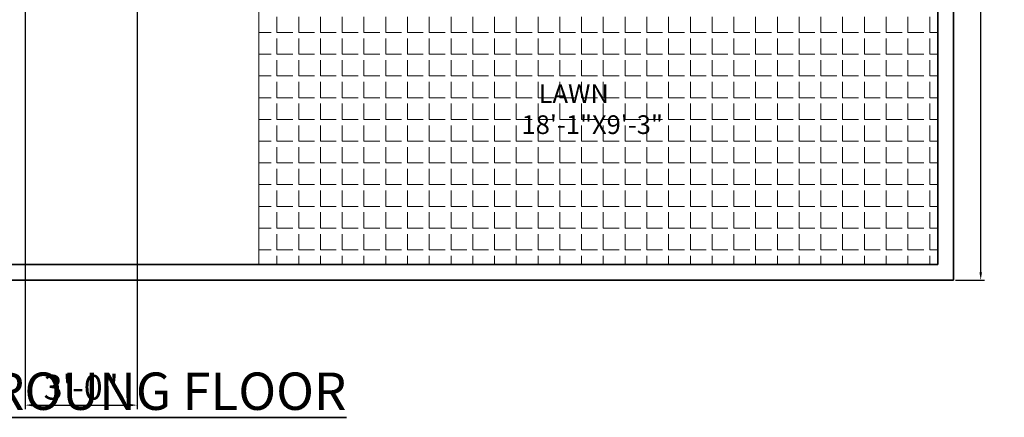
# Model space of a CAD drawing. Units: inches. Extents: x 1070 to 2371, y 645 to 1546.
# Tile 2 of 10: x 1342 to 1658, y 645 to 772. Entities that reach past the tile are written whole.
import ezdxf

# ---------------------------------------------------------------- set-up
doc = ezdxf.new("R2010")
doc.units = ezdxf.units.IN
for name, color, linetype, lineweight in [('A-ANNO-DIMS', 2, 'Continuous', 18), ('A-ANNO-TITL', 7, 'Continuous', 35), ('A-AREA-IDEN', 7, 'Continuous', 18), ('C-PROP', 7, 'Continuous', 35), ('L-PLNT-BEDS', 3, 'Continuous', 18), ('L-TURF-PATT', 9, 'Continuous', 13)]:
    doc.layers.add(name, color=color, linetype=linetype, lineweight=lineweight)
doc.styles.get("Standard").update_dxf_attribs({"font": 'arial.ttf'})
doc.dimstyles.new('ISO-25', dxfattribs={"dimtxt": 8, "dimasz": 2.5, "dimexe": 1.25, "dimexo": 0.625, "dimtad": 1, "dimtih": 1, "dimtoh": 1, "dimdec": 1, "dimlunit": 3, "dimtxsty": 'Standard', "dimcen": 2.5, "dimadec": 0, "dimazin": 0, "dimtfac": 1, "dimtdec": 1, "dimtmove": 0, "dimatfit": 3, "dimfxl": 1, "dimarcsym": 0})

# ---------------------------------------------------------------- blocks, each defined once
blk = doc.blocks.new('*D12')
at = {"layer": 'A-ANNO-DIMS', "color": 0, "lineweight": -2, "transparency": 16777216}
for p, q in [((1642.74, 1408.77), (1652.12, 1408.77)), ((1650.87, 1406.27), (1650.87, 1053.48)), ((1650.87, 691.27), (1650.87, 1044.06)), ((1642.74, 688.77), (1652.12, 688.77))]:
    blk.add_line(p, q, dxfattribs=at)
at = {"layer": 'A-ANNO-DIMS', "color": 0, "transparency": 16777216}
for points in [[(1650.46, 1406.27), (1651.29, 1406.27), (1650.87, 1408.77)], [(1650.46, 691.27), (1651.29, 691.27), (1650.87, 688.77)]]:
    blk.add_solid(points, dxfattribs=at)
at = {"layer": 'Defpoints', "color": 0, "transparency": 16777216}
for p in [(1642.11, 1408.77), (1642.11, 688.77), (1650.87, 688.77)]:
    blk.add_point(p, dxfattribs=at)
at = {"layer": 'A-ANNO-DIMS', "color": 0, "transparency": 16777216, "insert": (1650.87, 1048.77), "char_height": 8, "attachment_point": 5}
blk.add_mtext("60'", dxfattribs=at)
blk = doc.blocks.new('*D49')
at = {"layer": 'A-ANNO-DIMS', "color": 0, "lineweight": -2, "transparency": 16777216}
for p, q in [((1344.11, 1342.15), (1344.11, 647.32)), ((1380.11, 1342.15), (1380.11, 647.32)), ((1346.61, 648.57), (1377.61, 648.57))]:
    blk.add_line(p, q, dxfattribs=at)
at = {"layer": 'A-ANNO-DIMS', "color": 0, "transparency": 16777216}
for points in [[(1346.61, 648.99), (1346.61, 648.16), (1344.11, 648.57)], [(1377.61, 648.99), (1377.61, 648.16), (1380.11, 648.57)]]:
    blk.add_solid(points, dxfattribs=at)
at = {"layer": 'Defpoints', "color": 0, "transparency": 16777216}
for p in [(1344.11, 1342.77), (1380.11, 1342.77), (1380.11, 648.57)]:
    blk.add_point(p, dxfattribs=at)
at = {"layer": 'A-ANNO-DIMS', "color": 0, "transparency": 16777216, "insert": (1362.11, 653.28), "char_height": 8, "attachment_point": 5}
blk.add_mtext('3\'-0"', dxfattribs=at)

msp = doc.modelspace()

# ---------------------------------------------------------------- hatches: boundary and pattern name
at = {"layer": 'L-TURF-PATT'}
h = msp.add_hatch(dxfattribs=at)
h.set_pattern_fill('ANGLE', color=256)
h.set_pattern_definition([(0, (0, 0), (0, 6.985), [5.08, -1.905]), (90, (0, 0), (-6.985, 4e-16), [5.08, -1.905])])
h.paths.add_polyline_path([(1461.11, 804.77), (1419.11, 804.77), (1419.11, 693.77), (1637.11, 693.77), (1637.11, 804.77), (1600.11, 804.77)])
h.paths.add_polyline_path([(1501.06, 732.44), (1547.69, 732.44), (1547.69, 754.83), (1501.06, 754.83)], flags=24)

# ---------------------------------------------------------------- linework, layer by layer
at = {"layer": 'C-PROP'}
for p, q in [((1642.11, 1408.77), (1642.11, 688.77)), ((1637.11, 1403.77), (1637.11, 693.77)), ((1167.11, 693.77), (1637.11, 693.77)), ((1162.11, 688.77), (1642.11, 688.77))]:
    msp.add_line(p, q, dxfattribs=at)
at = {"layer": 'L-PLNT-BEDS'}
msp.add_line((1419.11, 804.77), (1419.11, 693.77), dxfattribs=at)

# ---------------------------------------------------------------- texts
at = {"layer": 'A-ANNO-TITL', "insert": (1322.21, 659.05), "char_height": 12, "attachment_point": 1}
msp.add_mtext_dynamic_manual_height_columns('{\\LGROUNG FLOOR }', width=357.2187, gutter_width=12.5, heights=[0], dxfattribs=at)
at = {"layer": 'A-AREA-IDEN', "insert": (1503.47, 751.74), "char_height": 6, "attachment_point": 1}
msp.add_mtext_dynamic_manual_height_columns('   LAWN\\P18\'-1"X9\'-3"', width=62.3796, gutter_width=12.5, heights=[0], dxfattribs=at)

# ---------------------------------------------------------------- dimensions: what is measured, and where the dimension line sits
at = {"layer": 'A-ANNO-DIMS'}
dim = msp.add_linear_dim(base=(1650.87, 688.77), p1=(1642.11, 1408.77), p2=(1642.11, 688.77), angle=90, dimstyle='ISO-25', override={"dimclrd": 0, "dimclre": 0, "dimclrt": 0}, dxfattribs=at)
dim.commit()
dim.dimension.update_dxf_attribs({"geometry": '*D12', "text_midpoint": (1650.87, 1048.77)})
dim = msp.add_linear_dim(base=(1380.11, 648.57), p1=(1344.11, 1342.77), p2=(1380.11, 1342.77), dimstyle='ISO-25', override={"dimdec": 1, "dimlfac": 1, "dimrnd": 0, "dimzin": 1, "dimdsep": 46, "dimlunit": 4, "dimfrac": 2}, dxfattribs=at)
dim.commit()
dim.dimension.update_dxf_attribs({"geometry": '*D49', "text_midpoint": (1362.11, 653.28)})

doc.saveas('drawing.dxf')
